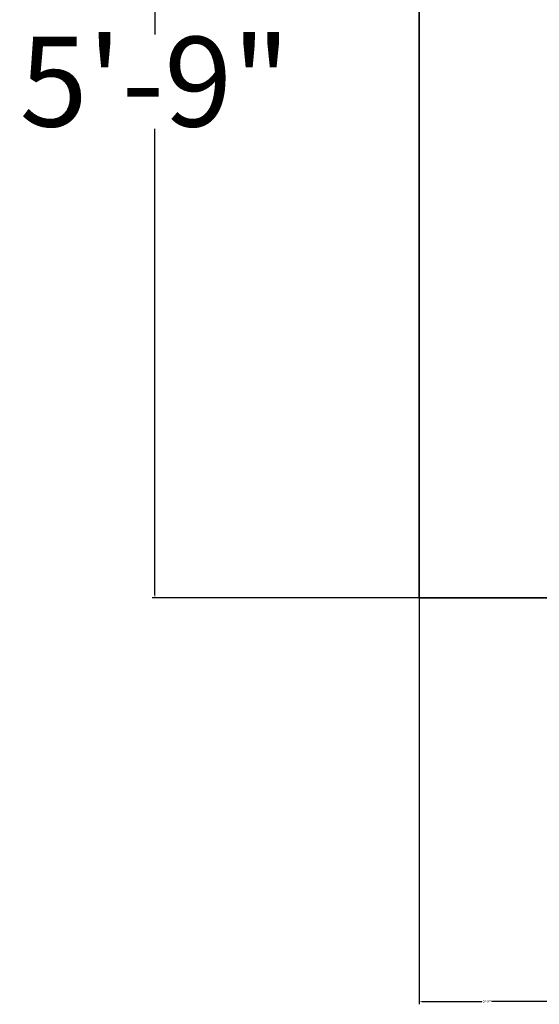
# Model space of a CAD drawing. Units: inches. Extents: x -5 to 330, y -522 to 40.
# Tile 1 of 23: x -3 to 32, y -522 to -457. Entities that reach past the tile are written whole.
import ezdxf

# ---------------------------------------------------------------- set-up
doc = ezdxf.new("R2010")
doc.units = ezdxf.units.IN
doc.header["$MEASUREMENT"] = 0
for name, color, linetype, lineweight in [('A-ANNO-DIMS', 2, 'Continuous', 18), ('A-SITE-WALL', 7, 'Continuous', 35), ('A-WALL', 7, 'Continuous', 35)]:
    doc.layers.add(name, color=color, linetype=linetype, lineweight=lineweight)
doc.styles.get("Standard").update_dxf_attribs({"font": 'arial.ttf'})
doc.dimstyles.get("Standard").update_dxf_attribs({"dimtxt": 0.18, "dimasz": 0.18, "dimexe": 0.18, "dimexo": 0.0625, "dimgap": 0.09, "dimtad": 0, "dimtih": 1, "dimtoh": 1, "dimdec": 0, "dimzin": 0, "dimdsep": 46, "dimlunit": 3, "dimtxsty": 'Standard', "dimcen": 0.09, "dimadec": 0, "dimazin": 0, "dimtfac": 1, "dimtdec": 0, "dimtofl": 0, "dimtmove": 0, "dimatfit": 3, "dimfxl": 1, "dimtolj": 1, "dimtzin": 0, "dimarcsym": 0})

# ---------------------------------------------------------------- blocks, each defined once
blk = doc.blocks.new('*D3')
at = {"layer": 'A-ANNO-DIMS', "color": 0, "lineweight": -2, "transparency": 16777216}
for p, q in [((23.447, -426.144), (5.666, -426.144)), ((5.846, -426.324), (5.846, -457.49)), ((5.846, -494.964), (5.846, -463.797)), ((23.447, -495.144), (5.666, -495.144))]:
    blk.add_line(p, q, dxfattribs=at)
at = {"layer": 'A-ANNO-DIMS', "color": 0, "transparency": 16777216}
for points in [[(5.816, -426.324), (5.876, -426.324), (5.846, -426.144)], [(5.816, -494.964), (5.876, -494.964), (5.846, -495.144)]]:
    blk.add_solid(points, dxfattribs=at)
at = {"layer": 'Defpoints', "color": 0, "transparency": 16777216}
for p in [(23.51, -426.144), (5.846, -495.144), (23.51, -495.144)]:
    blk.add_point(p, dxfattribs=at)
at = {"layer": 'A-ANNO-DIMS', "color": 0, "transparency": 16777216, "insert": (5.846, -460.644), "char_height": 6, "attachment_point": 5}
blk.add_mtext('\\A1;5\'-9"', dxfattribs=at)
blk = doc.blocks.new('*D50')
at = {"layer": 'A-ANNO-DIMS', "color": 0, "lineweight": -2, "transparency": 16777216}
for p, q in [((32.51, -417.206), (32.51, -522.309)), ((23.51, -426.206), (23.51, -522.309)), ((23.69, -522.129), (27.681, -522.129)), ((32.33, -522.129), (28.339, -522.129))]:
    blk.add_line(p, q, dxfattribs=at)
at = {"layer": 'A-ANNO-DIMS', "color": 0, "transparency": 16777216}
for points in [[(23.69, -522.099), (23.69, -522.159), (23.51, -522.129)], [(32.33, -522.099), (32.33, -522.159), (32.51, -522.129)]]:
    blk.add_solid(points, dxfattribs=at)
at = {"layer": 'Defpoints', "color": 0, "transparency": 16777216}
for p in [(32.51, -417.144), (23.51, -426.144), (32.51, -522.129)]:
    blk.add_point(p, dxfattribs=at)
at = {"layer": 'A-ANNO-DIMS', "color": 0, "transparency": 16777216, "insert": (28.01, -522.129), "char_height": 0.18, "attachment_point": 5}
blk.add_mtext('\\A1;0\'-9"', dxfattribs=at)

msp = doc.modelspace()

# ---------------------------------------------------------------- linework, layer by layer
at = {"layer": 'A-SITE-WALL'}
msp.add_line((23.51, -495.144), (281.01, -495.144), dxfattribs=at)
at = {"layer": 'A-WALL'}
msp.add_line((23.51, 12.356), (23.51, -495.144), dxfattribs=at)

# ---------------------------------------------------------------- dimensions: what is measured, and where the dimension line sits
at = {"layer": 'A-ANNO-DIMS'}
dim = msp.add_linear_dim(base=(32.51, -522.129), p1=(23.51, -426.144), p2=(32.51, -417.144), dimstyle='Standard', override={"dimdec": 1, "dimlfac": 1, "dimrnd": 0, "dimzin": 1, "dimdsep": 46, "dimlunit": 4, "dimfrac": 2}, dxfattribs=at)
dim.commit()
dim.dimension.update_dxf_attribs({"geometry": '*D50', "text_midpoint": (28.01, -522.129)})
dim = msp.add_linear_dim(base=(5.846, -495.144), p1=(23.51, -426.144), p2=(23.51, -495.144), angle=90, dimstyle='Standard', override={"dimtxt": 6, "dimclrd": 0, "dimclre": 0, "dimclrt": 0}, dxfattribs=at)
dim.commit()
dim.dimension.update_dxf_attribs({"geometry": '*D3', "text_midpoint": (5.846, -460.644)})

doc.saveas('drawing.dxf')
